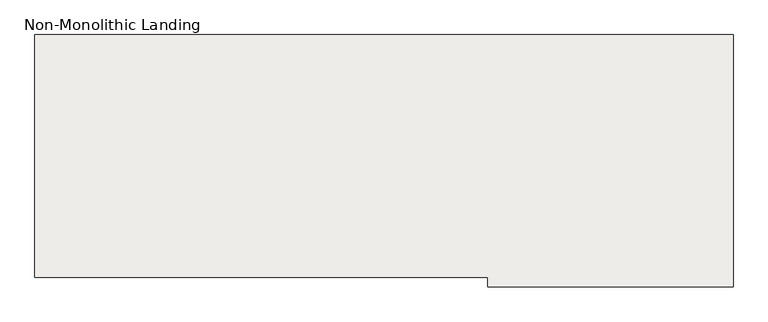
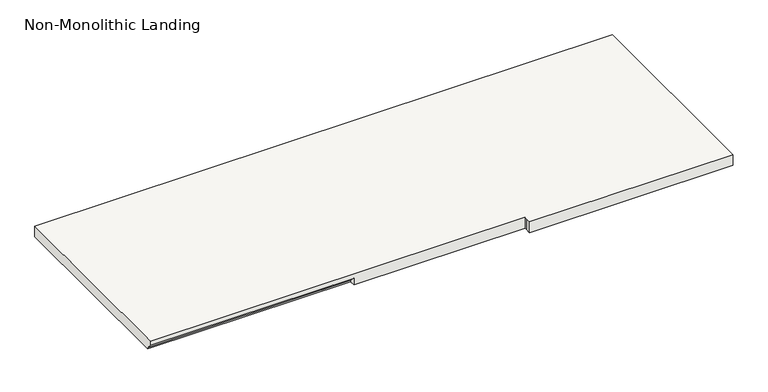
"""IFC4 building model written with IfcOpenShell, lengths in millimetres: slab geometry, Non-Monolithic Landing."""

from ifc_helpers import new_model, si_unit, origin, place, context, project, spatial, faceted_brep, source, transform, mapped, element, save


def non_monolithic_landing_fd591c5a(model_context):
    return source(origin(), model_context, "Body", "Brep", [
        faceted_brep([(-7448.5867944, 13309.8230289, 3409.95), (-7448.5867944, 13335.2230289, 3384.55), (-6534.1867944, 13335.2230289, 3384.55), (-6534.1867944, 13309.8230289, 3409.95), (-5762.1737939, 13309.8230289, 3429.0), (-5762.1737939, 13300.0419954, 3429.0), (-5762.1737939, 13274.6419954, 3429.0), (-4847.7737939, 13274.6419954, 3429.0), (-4847.7737939, 13300.0419954, 3429.0), (-4847.7737939, 14214.4419954, 3429.0), (-7448.5867944, 14214.4419954, 3429.0), (-7448.5867944, 13309.8230289, 3429.0), (-6534.1867944, 13335.2230289, 3378.2), (-7448.5867944, 13335.2230289, 3378.2), (-7448.5867944, 14214.4419954, 3378.2), (-4847.7737939, 14214.4419954, 3378.2), (-4847.7737939, 13300.0419954, 3378.2), (-4847.7737939, 13274.6419954, 3378.2), (-5762.1737939, 13274.6419954, 3378.2), (-5762.1737939, 13300.0419954, 3378.2), (-5762.1737939, 13309.8230289, 3378.2), (-6534.1867944, 13309.8230289, 3378.2)], [[[0, 1, 2, 3]], [[4, 5, 6, 7, 8, 9, 10, 11]], [[12, 13, 14, 15, 16, 17, 18, 19, 20, 21]], [[13, 12, 2, 1]], [[4, 11, 0, 3, 21, 20]], [[5, 4, 20, 19]], [[6, 5, 19, 18]], [[7, 6, 18, 17]], [[8, 7, 17, 16]], [[9, 8, 16, 15]], [[10, 9, 15, 14]], [[11, 10, 14, 13, 1, 0]], [[12, 21, 3, 2]]]),
    ])


if __name__ == "__main__":
    model = new_model("IFC4")
    model_context = context("Model", 3, world=origin())
    ifc_project = project(units=[si_unit("LENGTHUNIT", "METRE", prefix="MILLI")], contexts=[model_context])
    site = spatial("IfcSite", under=ifc_project)
    building = spatial("IfcBuilding", under=site)
    placement = place(None, origin())
    non_monolithic_landing_shape = non_monolithic_landing_fd591c5a(model_context)
    element("IfcSlab", 1, ObjectType="Non-Monolithic Landing", at=placement, inside=building, context=model_context, shape_type="MappedRepresentation", body=[
        mapped(non_monolithic_landing_shape, transform((0.0, 0.0, 0.0), x_axis=(1.0, 0.0, 0.0), y_axis=(0.0, 1.0, 0.0), z_axis=(0.0, 0.0, 1.0))),
    ])
    save(model, "model.ifc")
